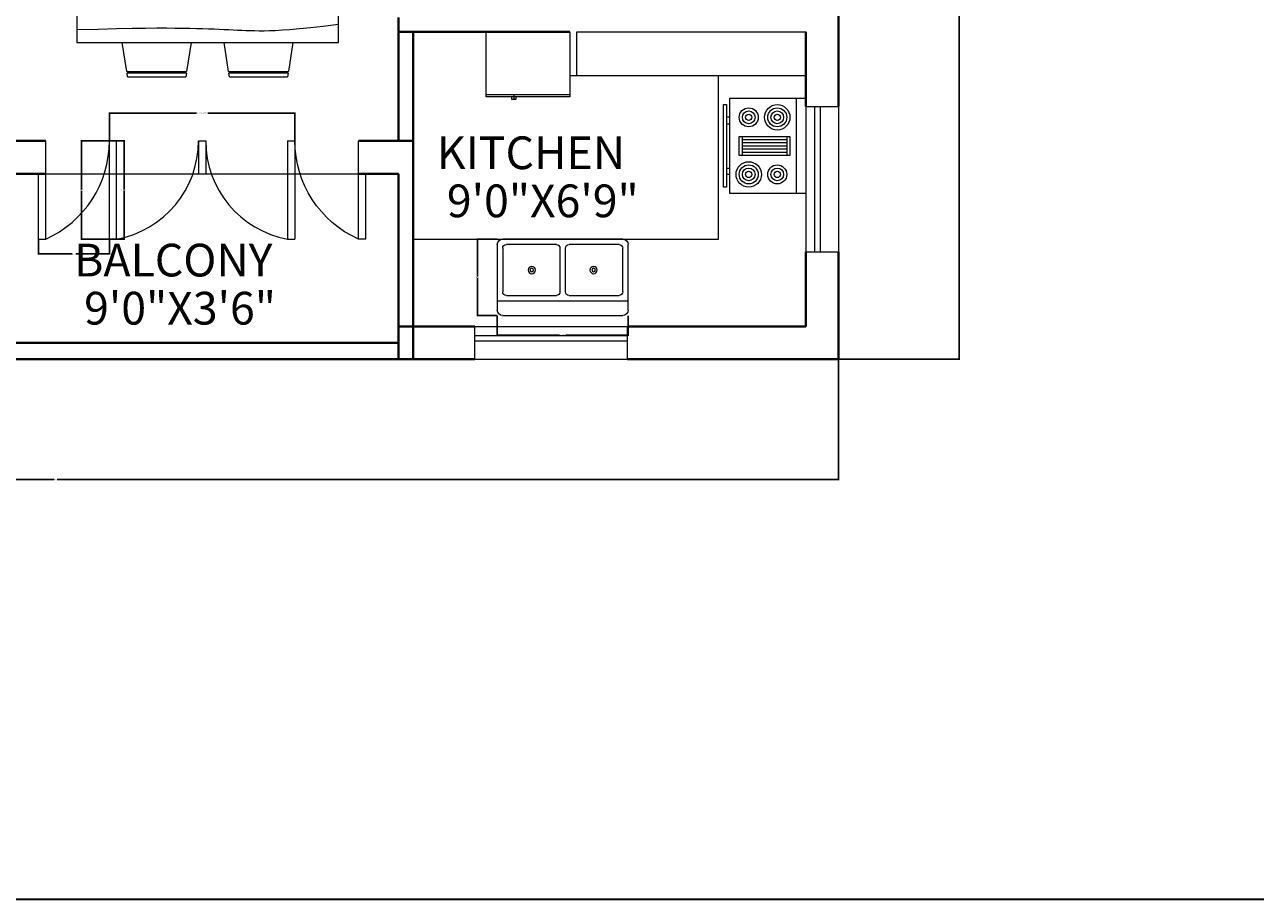
# Model space of a CAD drawing. Units: inches. Extents: x 2220 to 3422, y 783 to 1748.
# Tile 2 of 7: x 2483 to 2821, y 783 to 1023. Entities that reach past the tile are written whole.
import ezdxf

# ---------------------------------------------------------------- set-up
doc = ezdxf.new("R2010")
doc.units = ezdxf.units.IN
for name, color, linetype, lineweight in [('A-ANNO-DIMS', 2, 'Continuous', 18), ('A-ANNO-TTLB', 7, 'Continuous', 35), ('A-AREA-IDEN', 7, 'Continuous', 18), ('A-DOOR', 3, 'Continuous', 20), ('A-EQPM', 9, 'Continuous', 18), ('A-FLOR-CASE', 8, 'Continuous', 18), ('A-FLOR-FIXT', 9, 'Continuous', 18), ('A-FURN', 8, 'Continuous', 18), ('A-GLAZ', 4, 'Continuous', 18), ('A-WALL', 7, 'Continuous', 40)]:
    doc.layers.add(name, color=color, linetype=linetype, lineweight=lineweight)
doc.styles.get("Standard").update_dxf_attribs({"font": 'arial.ttf'})
doc.dimstyles.get("Standard").update_dxf_attribs({"dimtxt": 0.18, "dimasz": 0.18, "dimexe": 0.18, "dimexo": 0.0625, "dimgap": 0.09, "dimtad": 0, "dimtih": 1, "dimtoh": 1, "dimdec": 4, "dimzin": 0, "dimdsep": 46, "dimtxsty": 'Standard', "dimcen": 0.09, "dimadec": 0, "dimazin": 0, "dimtfac": 1, "dimtdec": 4, "dimtofl": 0, "dimtmove": 0, "dimatfit": 3, "dimfxl": 1, "dimtolj": 1, "dimtzin": 0, "dimarcsym": 0})

# ---------------------------------------------------------------- blocks, each defined once
blk = doc.blocks.new('Range-Oven - 30 in top')
for p, q in [((0, -3), (30, -3)), ((12, -6), (18, -6)), ((13, -20), (13, -6)), ((14, -6), (14, -20)), ((15, -20), (15, -6)), ((16, -6), (16, -20)), ((17, -20), (17, -6)), ((18, -20), (12, -20)), ((6, -24), (6, -25)), ((8, -25), (8, -24)), ((22, -25), (22, -24)), ((24, -24), (24, -25))]:
    blk.add_line(p, q)
for points in [[(0, -24), (0, 0), (30, 0), (30, -24)], [(12, -21), (12, -5), (18, -5), (18, -21)], [(2, -26), (2, -25), (28, -25), (28, -26)]]:
    blk.add_lwpolyline(points, close=True)
for centre, radius in [((6, -9), 4), ((6, -9), 3), ((6, -9), 2), ((24, -9), 3), ((24, -9), 2), ((6, -9), 1), ((24, -9), 1), ((6, -18), 3), ((24, -18), 4), ((24, -18), 3), ((6, -18), 2), ((6, -18), 1), ((24, -18), 2), ((24, -18), 1)]:
    blk.add_circle(centre, radius)
blk = doc.blocks.new('Refrigerator-2 door - 36 in top')
for p, q in [((0, -26.999999), (36, -26.999999)), ((11, -27.999999), (11, -28.999999)), ((11, -28.999999), (13, -28.999999)), ((12, -26.999999), (12, -28.999999)), ((13, -28.999999), (13, -27.999999))]:
    blk.add_line(p, q)
blk.add_lwpolyline([(0, -27.999999), (0, 0), (36, 0), (36, -27.999999)], close=True)
blk = doc.blocks.new('Sink-double - 36 in top')
for p, q in [((-18, -4), (18, -4)), ((-0.75, -18.5), (-0.75, -6.5)), ((0.75, -6.5), (0.75, -18.5))]:
    blk.add_line(p, q)
for points in [[(-16.5, 0), (16.5, 0)], [(-18, -19.5), (-18, -1.5)], [(18, -1.5), (18, -19.5)], [(-16.5, -18.5), (-16.5, -6.5)], [(-15.5, -5.5), (-1.75, -5.5)], [(1.75, -5.5), (15.5, -5.5)], [(16.5, -6.5), (16.5, -18.5)], [(-1.75, -19.5), (-15.5, -19.5)], [(15.5, -19.5), (1.75, -19.5)], [(16.5, -21), (-16.5, -21)]]:
    blk.add_lwpolyline(points)
for centre, radius in [((-8.5, -12.5), 1), ((-8.5, -12.5), 0.5), ((8.5, -12.5), 1), ((8.5, -12.5), 0.5)]:
    blk.add_circle(centre, radius)
for centre, radius, start, end in [((-16.5, -1.5), 1.5, 90, 180), ((16.5, -1.5), 1.5, 0, 90), ((-15.5, -6.5), 1, 90, 180), ((-1.75, -6.5), 1, 0, 90), ((1.75, -6.5), 1, 90, 180), ((15.5, -6.5), 1, 0, 90), ((-16.5, -19.5), 1.5, 180, 270), ((-15.5, -18.5), 1, 180, 270), ((-1.75, -18.5), 1, 270, 0), ((1.75, -18.5), 1, 180, 270), ((15.5, -18.5), 1, 270, 0), ((16.5, -19.5), 1.5, 270, 0)]:
    blk.add_arc(centre, radius, start, end)
blk = doc.blocks.new('Dining Set - 36 x 72 in.')
for p, q in [((-22, 27.5), (-22.1562, 26.50042)), ((-22, 27.5), (-6, 27.5)), ((-5.8437, 26.49966), (-6, 27.5)), ((6, 27.5), (5.8438, 26.50042)), ((6, 27.5), (22, 27.5)), ((22.1563, 26.49966), (22, 27.5)), ((-22.2343, 26.00059), (-23.4847, 17.99762)), ((-22.2304, 26), (-5.7608, 26)), ((-5.8416, 26.5), (-22.1534, 26.5)), ((-4.5152, 17.99762), (-5.7655, 25.99926)), ((5.7657, 26.00059), (4.5153, 17.99762)), ((5.7696, 26), (22.2392, 26)), ((22.1584, 26.5), (5.8466, 26.5)), ((23.4848, 17.99762), (22.2345, 25.99926)), ((36, 18), (-36, 18)), ((-36, 18), (-36, -18)), ((36, -18), (36, 18)), ((-45.5, 8), (-44.5004, 8.15617)), ((-45.5, 8), (-45.5, -8)), ((-44.5, -8.15843), (-44.5, 8.15338)), ((-44.0006, 8.23428), (-35.9976, 9.48474)), ((-44, 8.23041), (-44, -8.23915)), ((44.0006, 8.23428), (35.9976, 9.48474)), ((44, 8.23041), (44, -8.23915)), ((44.5, -8.15843), (44.5, 8.15338)), ((45.5, 8), (44.5005, 8.15617)), ((45.5, 8), (45.5, -8)), ((-44.4997, -8.15631), (-45.5, -8)), ((-35.9976, -9.48476), (-43.9993, -8.2345)), ((35.9976, -9.48476), (43.9993, -8.2345)), ((44.4997, -8.15631), (45.5, -8)), ((-36, -18), (36, -18)), ((-22.2343, -26.0006), (-23.4847, -17.99762)), ((-4.5152, -17.99762), (-5.7655, -25.99928)), ((5.7657, -26.0006), (4.5153, -17.99762)), ((23.4848, -17.99762), (22.2345, -25.99928)), ((-22.2304, -26), (-5.7608, -26)), ((-22, -27.5), (-22.1562, -26.50044)), ((-5.8416, -26.5), (-22.1534, -26.5)), ((-5.8437, -26.49967), (-6, -27.5)), ((5.7696, -26), (22.2392, -26)), ((6, -27.5), (5.8438, -26.50044)), ((22.1584, -26.5), (5.8466, -26.5)), ((22.1563, -26.49967), (22, -27.5)), ((-22, -27.5), (-6, -27.5)), ((6, -27.5), (22, -27.5))]:
    blk.add_line(p, q)
for points in [[(-36, 15), (-31.1772, 14.97754), (-26.8079, 14.91406), (-22.8538, 14.81543), (-19.276, 14.6875), (-16.0362, 14.53613), (-13.0957, 14.36718), (-10.4159, 14.18652), (-7.9583, 14), (-5.6904, 13.81315), (-3.6035, 13.63021), (-1.6954, 13.45508), (0.0365, 13.29166), (1.5945, 13.14388), (2.9811, 13.01562), (4.1988, 12.9108), (5.25, 12.83333), (6.1393, 12.78613), (6.8802, 12.76823), (7.4883, 12.77767), (7.9792, 12.8125), (8.3685, 12.87077), (8.6719, 12.95052), (8.9049, 13.0498), (9.0833, 13.16666), (9.2205, 13.29899), (9.3216, 13.44401), (9.3895, 13.59879), (9.4271, 13.76041), (9.4373, 13.92594), (9.4232, 14.09245), (9.3875, 14.257), (9.3333, 14.41666), (9.2638, 14.56917), (9.1836, 14.71484), (9.0975, 14.85465), (9.0104, 14.98958), (8.9272, 15.1206), (8.8529, 15.2487), (8.7922, 15.37483), (8.75, 15.5), (8.7305, 15.62467), (8.7344, 15.74739), (8.7617, 15.86621), (8.8125, 15.97916), (8.8867, 16.08431), (8.9844, 16.17968), (9.1055, 16.26334), (9.25, 16.33333), (9.4189, 16.38802), (9.6172, 16.42708), (9.8506, 16.45052), (10.125, 16.45833), (10.4463, 16.45052), (10.8203, 16.42708), (11.2529, 16.38802), (11.75, 16.33333), (12.3184, 16.26318), (12.9694, 16.17838), (13.7151, 16.07991), (14.5677, 15.96875), (15.5395, 15.84586), (16.6426, 15.71224), (17.8893, 15.56884), (19.2917, 15.41666), (20.859, 15.25667), (22.5879, 15.08984), (24.4721, 14.91715), (26.5052, 14.73958), (28.6809, 14.5581), (30.9929, 14.3737), (33.4347, 14.18733), (36, 14)], [(-36, 10), (-28.9766, 10.14274), (-23.1725, 10.20442), (-18.4241, 10.19775), (-14.5677, 10.13541), (-11.4399, 10.03011), (-8.877, 9.89453), (-6.7154, 9.74137), (-4.7917, 9.58333), (-2.9698, 9.43082), (-1.2246, 9.28515), (0.4415, 9.14534), (2.026, 9.01041), (3.5266, 8.87939), (4.9408, 8.7513), (6.266, 8.62516), (7.5, 8.5), (8.6411, 8.37549), (9.6914, 8.2539), (10.6538, 8.13818), (11.5312, 8.03125), (12.3267, 7.93603), (13.043, 7.85547), (13.6831, 7.79248), (14.25, 7.75), (14.7471, 7.7303), (15.1797, 7.73307), (15.5537, 7.75732), (15.875, 7.80208), (16.1494, 7.86637), (16.3828, 7.94922), (16.5811, 8.04964), (16.75, 8.16666), (16.8944, 8.29915), (17.0143, 8.44531), (17.1089, 8.60319), (17.1771, 8.77083), (17.218, 8.94629), (17.2305, 9.1276), (17.2137, 9.31282), (17.1667, 9.5), (17.0895, 9.6875), (16.987, 9.875), (16.8649, 10.0625), (16.7292, 10.25), (16.5856, 10.4375), (16.4401, 10.625), (16.2985, 10.8125), (16.1667, 11), (16.05, 11.18733), (15.9518, 11.3737), (15.8752, 11.5581), (15.8229, 11.73958), (15.798, 11.91715), (15.8034, 12.08984), (15.842, 12.25667), (15.9167, 12.41666), (16.0295, 12.56836), (16.1784, 12.70833), (16.3605, 12.83268), (16.5729, 12.9375), (16.8127, 13.01888), (17.0768, 13.07291), (17.3625, 13.0957), (17.6667, 13.08333), (17.9894, 13.03312), (18.3418, 12.94726), (18.7382, 12.82918), (19.1927, 12.68229), (19.7195, 12.51001), (20.3327, 12.31575), (21.0465, 12.10294), (21.875, 11.875), (22.8357, 11.63354), (23.959, 11.37304), (25.2786, 11.08618), (26.8282, 10.76562), (28.6414, 10.40405), (30.752, 9.99414), (33.1936, 9.52856), (36, 9)], [(-36, 5.5), (-30.7157, 5.3348), (-26.069, 5.20963), (-21.9946, 5.11767), (-18.4271, 5.05208), (-15.3009, 5.00602), (-12.5508, 4.97265), (-10.1112, 4.94515), (-7.9167, 4.91666), (-5.909, 4.88167), (-4.0586, 4.83984), (-2.3429, 4.79215), (-0.7396, 4.73958), (0.7739, 4.6831), (2.22, 4.6237), (3.6213, 4.56233), (5, 4.5), (6.373, 4.43782), (7.7344, 4.3776), (9.0723, 4.32129), (10.375, 4.27083), (11.6309, 4.22819), (12.8281, 4.19531), (13.9551, 4.17415), (15, 4.16666), (15.954, 4.17448), (16.819, 4.19791), (17.6001, 4.23698), (18.3021, 4.29166), (18.9299, 4.36198), (19.4883, 4.44791), (19.9823, 4.54948), (20.4167, 4.66666), (20.7969, 4.79899), (21.1302, 4.94401), (21.4245, 5.09879), (21.6875, 5.26041), (21.9271, 5.42594), (22.1511, 5.59245), (22.3672, 5.757), (22.5834, 5.91666), (22.8065, 6.06868), (23.0404, 6.21093), (23.2879, 6.34147), (23.5521, 6.45833), (23.8358, 6.55957), (24.142, 6.64323), (24.4735, 6.70735), (24.8334, 6.75), (25.2235, 6.76969), (25.642, 6.76692), (26.0858, 6.74267), (26.5521, 6.69791), (27.0379, 6.63362), (27.5404, 6.55078), (28.0565, 6.45036), (28.5834, 6.33333), (29.1242, 6.19987), (29.7071, 6.04687), (30.3661, 5.87044), (31.1354, 5.66666), (32.0493, 5.43164), (33.142, 5.16146), (34.4475, 4.85221), (36, 4.5)], [(-36, -1), (-30.7915, -0.6591), (-26.0195, -0.38216), (-21.6519, -0.16284), (-17.6563, 0.00521), (-14.0005, 0.12833), (-10.6523, 0.21289), (-7.5796, 0.26522), (-4.75, 0.29166), (-2.134, 0.29793), (0.2878, 0.28711), (2.5317, 0.26163), (4.6146, 0.22396), (6.5529, 0.17651), (8.3633, 0.12174), (10.0623, 0.06209), (11.6667, 0), (13.1899, -0.06201), (14.6341, -0.1211), (15.9982, -0.17432), (17.2813, -0.21875), (18.4823, -0.25147), (19.6003, -0.26953), (20.6343, -0.27002), (21.5834, -0.25), (22.4481, -0.20768), (23.2357, -0.14584), (23.9549, -0.06836), (24.6146, 0.02083), (25.2235, 0.11784), (25.7904, 0.21875), (26.3241, 0.31966), (26.8334, 0.41666), (27.3265, 0.50618), (27.8099, 0.58593), (28.2894, 0.65397), (28.7709, 0.70833), (29.2601, 0.74707), (29.763, 0.76823), (30.2855, 0.76985), (30.8334, 0.75), (31.4088, 0.70784), (31.9994, 0.64713), (32.589, 0.57275), (33.1615, 0.48958), (33.7008, 0.4025), (34.1908, 0.3164), (34.6153, 0.23616), (34.9584, 0.16666), (35.2099, 0.11165), (35.3848, 0.07031), (35.504, 0.04069), (35.5886, 0.02083), (35.6594, 0.00879), (35.7377, 0.0026), (35.8442, 0.00032), (36, 0)], [(-36, -6.5), (-27.1843, -6.31267), (-20.084, -6.1263), (-14.469, -5.9419), (-10.1094, -5.76042), (-6.7752, -5.58285), (-4.2363, -5.41016), (-2.2629, -5.24333), (-0.625, -5.08334), (0.8708, -4.93099), (2.2715, -4.78646), (3.5872, -4.64974), (4.8281, -4.52084), (6.0046, -4.39974), (7.127, -4.28646), (8.2053, -4.18099), (9.25, -4.08334), (10.2705, -3.99382), (11.2734, -3.91407), (12.2647, -3.84603), (13.25, -3.79167), (14.2354, -3.75293), (15.2266, -3.73177), (16.2295, -3.73015), (17.25, -3.75), (18.2912, -3.79248), (19.3451, -3.85547), (20.4009, -3.93604), (21.4479, -4.03125), (22.4754, -4.13819), (23.4727, -4.25391), (24.4289, -4.37549), (25.3334, -4.5), (26.1785, -4.62492), (26.9694, -4.74935), (27.7145, -4.87281), (28.4219, -4.99479), (29.1, -5.11483), (29.7572, -5.23242), (30.4016, -5.34709), (31.0417, -5.45834), (31.6837, -5.56437), (32.3262, -5.65821), (32.9658, -5.73153), (33.599, -5.77604), (34.2224, -5.78345), (34.8327, -5.74545), (35.4264, -5.65373), (36, -5.5)], [(-36, -10), (-26.4022, -9.81299), (-18.4675, -9.62891), (-11.9839, -9.45069), (-6.7396, -9.28125), (-2.5226, -9.12354), (0.8789, -8.98047), (3.6769, -8.85498), (6.0833, -8.75), (8.2767, -8.66765), (10.3021, -8.60677), (12.1712, -8.56543), (13.8958, -8.54167), (15.4876, -8.53353), (16.9583, -8.53907), (18.3197, -8.55632), (19.5834, -8.58334), (20.7616, -8.61841), (21.8685, -8.66081), (22.9188, -8.71004), (23.9271, -8.76563), (24.9081, -8.82707), (25.8763, -8.89388), (26.8465, -8.96558), (27.8334, -9.04167), (28.8474, -9.12118), (29.8828, -9.20117), (30.93, -9.27824), (31.9792, -9.34896), (33.0205, -9.40991), (34.0443, -9.45768), (35.0407, -9.48885), (36, -9.5)], [(-36, -14.5), (-30.0881, -14.33513), (-25.0332, -14.21224), (-20.7312, -14.12647), (-17.0781, -14.07292), (-13.97, -14.04671), (-11.3027, -14.04297), (-8.9724, -14.05681), (-6.875, -14.08334), (-4.9224, -14.11833), (-3.0905, -14.16016), (-1.3709, -14.20785), (0.2448, -14.26042), (1.7647, -14.3169), (3.1973, -14.3763), (4.5507, -14.43767), (5.8333, -14.5), (7.0554, -14.5621), (8.235, -14.62175), (9.3922, -14.67652), (10.5469, -14.72396), (11.7192, -14.76164), (12.929, -14.78711), (14.1965, -14.79794), (15.5417, -14.79167), (16.9933, -14.76424), (18.6152, -14.70508), (20.4804, -14.60197), (22.6615, -14.44271), (25.2312, -14.21509), (28.2624, -13.9069), (31.8277, -13.50594), (36, -13)]]:
    blk.add_lwpolyline(points)
blk = doc.blocks.new('DOOR-BALCONY-CENTER')
for p, q in [((0, 0), (0, 27)), ((0, 27), (2, 27)), ((2, 0), (2, 27)), ((24.5, 27), (24.5, 18)), ((24.5, 27), (26.5, 27)), ((26.5, 27), (26.5, 18)), ((49, 27), (49, 0)), ((49, 27), (51, 27)), ((51, 27), (51, 0)), ((0, 0), (2, 0)), ((49, 0), (51, 0))]:
    blk.add_line(p, q)
for centre, start, end in [((-2.95, 27), 280.3889, 0), ((53.95, 27), 180, 259.6111)]:
    blk.add_arc(centre, 27.45, start, end)
blk = doc.blocks.new('DOOR-BALCONY-END-A')
for p, q in [((2, 0), (2, 27)), ((0, 0), (0, 18)), ((0, 0), (2, 0))]:
    blk.add_line(p, q)
blk.add_arc((-10.08, 27), 29.58, 294.1016, 0)
blk = doc.blocks.new('*D29')
at = {"layer": 'A-ANNO-DIMS', "color": 0, "lineweight": -2, "transparency": 16777216}
for p, q in [((2612.7, 943.33), (2612.7, 937.81)), ((2648.7, 943.33), (2648.7, 937.81)), ((2612.88, 937.99), (2629.85, 937.99)), ((2648.52, 937.99), (2631.56, 937.99))]:
    blk.add_line(p, q, dxfattribs=at)
at = {"layer": 'A-ANNO-DIMS', "color": 0, "transparency": 16777216}
for points in [[(2612.88, 938.02), (2612.88, 937.96), (2612.7, 937.99)], [(2648.52, 938.02), (2648.52, 937.96), (2648.7, 937.99)]]:
    blk.add_solid(points, dxfattribs=at)
at = {"layer": 'Defpoints', "color": 0, "transparency": 16777216}
for p in [(2612.7, 943.39), (2648.7, 943.39), (2648.7, 937.99)]:
    blk.add_point(p, dxfattribs=at)
at = {"layer": 'A-ANNO-DIMS', "color": 0, "transparency": 16777216, "insert": (2630.7, 937.99), "char_height": 0.18, "attachment_point": 5}
blk.add_mtext('\\A1;SINK 36 TYP.', dxfattribs=at)
blk = doc.blocks.new('*D30')
at = {"layer": 'A-ANNO-DIMS', "color": 0, "lineweight": -2, "transparency": 16777216}
for p, q in [((2612.64, 964.39), (2607.12, 964.39)), ((2607.3, 964.21), (2607.3, 954.07)), ((2607.3, 943.57), (2607.3, 953.71)), ((2612.64, 943.39), (2607.12, 943.39))]:
    blk.add_line(p, q, dxfattribs=at)
at = {"layer": 'A-ANNO-DIMS', "color": 0, "transparency": 16777216}
for points in [[(2607.27, 964.21), (2607.33, 964.21), (2607.3, 964.39)], [(2607.27, 943.57), (2607.33, 943.57), (2607.3, 943.39)]]:
    blk.add_solid(points, dxfattribs=at)
at = {"layer": 'Defpoints', "color": 0, "transparency": 16777216}
for p in [(2612.7, 964.39), (2607.3, 943.39), (2612.7, 943.39)]:
    blk.add_point(p, dxfattribs=at)
at = {"layer": 'A-ANNO-DIMS', "color": 0, "transparency": 16777216, "insert": (2607.3, 953.89), "char_height": 0.18, "attachment_point": 5}
blk.add_mtext('\\A1;21 TYP.', dxfattribs=at)
blk = doc.blocks.new('*D43')
at = {"layer": 'A-ANNO-DIMS', "color": 0, "lineweight": -2, "transparency": 16777216}
for p, q in [((2506.05, 991.45), (2506.05, 999.22)), ((2506.23, 999.04), (2529.97, 999.04)), ((2556.87, 999.04), (2533.12, 999.04)), ((2557.05, 991.45), (2557.05, 999.22))]:
    blk.add_line(p, q, dxfattribs=at)
at = {"layer": 'A-ANNO-DIMS', "color": 0, "transparency": 16777216}
for points in [[(2506.23, 999.07), (2506.23, 999.01), (2506.05, 999.04)], [(2556.87, 999.07), (2556.87, 999.01), (2557.05, 999.04)]]:
    blk.add_solid(points, dxfattribs=at)
at = {"layer": 'Defpoints', "color": 0, "transparency": 16777216}
for p in [(2557.05, 999.04), (2506.05, 991.39), (2557.05, 991.39)]:
    blk.add_point(p, dxfattribs=at)
at = {"layer": 'A-ANNO-DIMS', "color": 0, "transparency": 16777216, "insert": (2531.55, 999.04), "char_height": 0.18, "attachment_point": 5}
blk.add_mtext('\\A1;BALCONY DOOR 51 TYP.', dxfattribs=at)
blk = doc.blocks.new('*D44')
at = {"layer": 'A-ANNO-DIMS', "color": 0, "lineweight": -2, "transparency": 16777216}
for p, q in [((2505.98, 991.39), (2498.22, 991.39)), ((2498.4, 991.21), (2498.4, 978.07)), ((2498.4, 964.57), (2498.4, 977.71)), ((2505.98, 964.39), (2498.22, 964.39))]:
    blk.add_line(p, q, dxfattribs=at)
at = {"layer": 'A-ANNO-DIMS', "color": 0, "transparency": 16777216}
for points in [[(2498.37, 991.21), (2498.43, 991.21), (2498.4, 991.39)], [(2498.37, 964.57), (2498.43, 964.57), (2498.4, 964.39)]]:
    blk.add_solid(points, dxfattribs=at)
at = {"layer": 'Defpoints', "color": 0, "transparency": 16777216}
for p in [(2498.4, 991.39), (2506.05, 991.39), (2506.05, 964.39)]:
    blk.add_point(p, dxfattribs=at)
at = {"layer": 'A-ANNO-DIMS', "color": 0, "transparency": 16777216, "insert": (2498.4, 977.89), "char_height": 0.18, "attachment_point": 5}
blk.add_mtext('\\A1;27 TYP.', dxfattribs=at)
blk = doc.blocks.new('*D45')
at = {"layer": 'A-ANNO-DIMS', "color": 0, "lineweight": -2, "transparency": 16777216}
for p, q in [((2506.11, 991.39), (2510.28, 991.39)), ((2510.1, 991.21), (2510.1, 978.07)), ((2510.1, 964.57), (2510.1, 977.71)), ((2506.11, 964.39), (2510.28, 964.39))]:
    blk.add_line(p, q, dxfattribs=at)
at = {"layer": 'A-ANNO-DIMS', "color": 0, "transparency": 16777216}
for points in [[(2510.07, 991.21), (2510.13, 991.21), (2510.1, 991.39)], [(2510.07, 964.57), (2510.13, 964.57), (2510.1, 964.39)]]:
    blk.add_solid(points, dxfattribs=at)
at = {"layer": 'Defpoints', "color": 0, "transparency": 16777216}
for p in [(2506.05, 991.39), (2510.1, 991.39), (2506.05, 964.39)]:
    blk.add_point(p, dxfattribs=at)
at = {"layer": 'A-ANNO-DIMS', "color": 0, "transparency": 16777216, "insert": (2510.1, 977.89), "char_height": 0.18, "attachment_point": 5}
blk.add_mtext('\\A1;END LEAF A 27 TYP.', dxfattribs=at)
blk = doc.blocks.new('*D46')
at = {"layer": 'A-ANNO-DIMS', "color": 0, "lineweight": -2, "transparency": 16777216}
for p, q in [((2486.55, 964.33), (2486.55, 960.16)), ((2506.05, 964.33), (2506.05, 960.16)), ((2486.73, 960.34), (2495.77, 960.34)), ((2505.87, 960.34), (2496.83, 960.34))]:
    blk.add_line(p, q, dxfattribs=at)
at = {"layer": 'A-ANNO-DIMS', "color": 0, "transparency": 16777216}
for points in [[(2486.73, 960.37), (2486.73, 960.31), (2486.55, 960.34)], [(2505.87, 960.37), (2505.87, 960.31), (2506.05, 960.34)]]:
    blk.add_solid(points, dxfattribs=at)
at = {"layer": 'Defpoints', "color": 0, "transparency": 16777216}
for p in [(2486.55, 964.39), (2506.05, 964.39), (2506.05, 960.34)]:
    blk.add_point(p, dxfattribs=at)
at = {"layer": 'A-ANNO-DIMS', "color": 0, "transparency": 16777216, "insert": (2496.3, 960.34), "char_height": 0.18, "attachment_point": 5}
blk.add_mtext('\\A1;20 TYP.', dxfattribs=at)
blk = doc.blocks.new('*D53')
at = {"layer": 'A-ANNO-DIMS', "color": 0, "lineweight": -2, "transparency": 16777216}
for p, q in [((2276.05, 931.33), (2276.05, 898.06)), ((2706.55, 931.33), (2706.55, 898.06)), ((2276.23, 898.24), (2490.9, 898.24)), ((2706.37, 898.24), (2491.69, 898.24))]:
    blk.add_line(p, q, dxfattribs=at)
at = {"layer": 'A-ANNO-DIMS', "color": 0, "transparency": 16777216}
for points in [[(2276.23, 898.27), (2276.23, 898.21), (2276.05, 898.24)], [(2706.37, 898.27), (2706.37, 898.21), (2706.55, 898.24)]]:
    blk.add_solid(points, dxfattribs=at)
at = {"layer": 'Defpoints', "color": 0, "transparency": 16777216}
for p in [(2276.05, 931.39), (2706.55, 931.39), (2706.55, 898.24)]:
    blk.add_point(p, dxfattribs=at)
at = {"layer": 'A-ANNO-DIMS', "color": 0, "transparency": 16777216, "insert": (2491.3, 898.24), "char_height": 0.18, "attachment_point": 5}
blk.add_mtext('\\A1;430.5', dxfattribs=at)
blk = doc.blocks.new('*D57')
at = {"layer": 'A-ANNO-DIMS', "color": 0, "lineweight": -2, "transparency": 16777216}
for p, q in [((2706.61, 1218.39), (2739.88, 1218.39)), ((2739.7, 1218.21), (2739.7, 1075.07)), ((2739.7, 931.57), (2739.7, 1074.71)), ((2706.61, 931.39), (2739.88, 931.39))]:
    blk.add_line(p, q, dxfattribs=at)
at = {"layer": 'A-ANNO-DIMS', "color": 0, "transparency": 16777216}
for points in [[(2739.67, 1218.21), (2739.73, 1218.21), (2739.7, 1218.39)], [(2739.67, 931.57), (2739.73, 931.57), (2739.7, 931.39)]]:
    blk.add_solid(points, dxfattribs=at)
at = {"layer": 'Defpoints', "color": 0, "transparency": 16777216}
for p in [(2706.55, 1218.39), (2706.55, 931.39), (2739.7, 931.39)]:
    blk.add_point(p, dxfattribs=at)
at = {"layer": 'A-ANNO-DIMS', "color": 0, "transparency": 16777216, "insert": (2739.7, 1074.89), "char_height": 0.18, "attachment_point": 5}
blk.add_mtext('\\A1;287', dxfattribs=at)

msp = doc.modelspace()

# ---------------------------------------------------------------- linework, layer by layer
at = {"layer": 'A-ANNO-TTLB'}
msp.add_lwpolyline([(2220.0037, 1747.9465), (3422.343, 1747.9465), (3422.343, 782.804), (2220.0037, 782.804)], close=True, dxfattribs=at)
at = {"layer": 'A-DOOR'}
msp.add_line((2488.5466, 982.3907), (2574.5466, 982.3907), dxfattribs=at)
at = {"layer": 'A-FLOR-CASE'}
for p, q in [((2632.6148, 1021.3907), (2632.6148, 1009.3907)), ((2634.5466, 1009.3907), (2634.5466, 1021.3907)), ((2634.5466, 1021.3907), (2697.5466, 1021.3907)), ((2632.6148, 1009.3907), (2697.5466, 1009.3907)), ((2673.5466, 964.3907), (2673.5466, 1009.3907)), ((2589.5466, 964.3907), (2673.5466, 964.3907))]:
    msp.add_line(p, q, dxfattribs=at)
at = {"layer": 'A-GLAZ'}
for p, q in [((2697.5466, 1000.8907), (2706.5466, 1000.8907)), ((2697.5466, 1000.8907), (2697.5466, 960.8907)), ((2700.0466, 960.8907), (2700.0466, 1000.8907)), ((2701.5466, 960.8907), (2701.5466, 1000.8907)), ((2706.5466, 1000.8907), (2706.5466, 960.8907)), ((2697.5466, 960.8907), (2706.5466, 960.8907)), ((2606.5466, 931.3907), (2606.5466, 940.3907)), ((2606.5466, 940.3907), (2648.5466, 940.3907)), ((2606.5466, 937.8907), (2648.5466, 937.8907)), ((2648.5466, 931.3907), (2648.5466, 940.3907)), ((2606.5466, 936.3907), (2648.5466, 936.3907)), ((2606.5466, 931.3907), (2648.5466, 931.3907))]:
    msp.add_line(p, q, dxfattribs=at)
at = {"layer": 'A-WALL'}
for p, q in [((2706.5466, 1000.8907), (2706.5466, 1037.3907)), ((2585.5466, 1021.3907), (2585.5466, 1025.3907)), ((2585.5466, 1021.3907), (2632.6148, 1021.3907)), ((2585.5466, 1021.3907), (2585.5466, 991.3907)), ((2589.5466, 991.3907), (2589.5466, 1021.3907)), ((2697.5466, 1000.8907), (2697.5466, 1021.3907)), ((2477.5466, 991.3907), (2488.5466, 991.3907)), ((2574.5466, 991.3907), (2589.5466, 991.3907)), ((2589.5466, 931.3907), (2589.5466, 991.3907)), ((2477.5466, 982.3907), (2488.5466, 982.3907)), ((2574.5466, 982.3907), (2585.5466, 982.3907)), ((2585.5466, 931.3907), (2585.5466, 982.3907)), ((2697.5466, 940.3907), (2697.5466, 960.8907)), ((2706.5466, 931.3907), (2706.5466, 960.8907)), ((2585.5466, 940.3907), (2606.5466, 940.3907)), ((2648.5466, 940.3907), (2697.5466, 940.3907)), ((2477.5466, 935.8907), (2585.5466, 935.8907)), ((2477.5466, 931.3907), (2585.5466, 931.3907)), ((2585.5466, 931.3907), (2589.5466, 931.3907)), ((2589.5466, 931.3907), (2606.5466, 931.3907)), ((2648.5466, 931.3907), (2706.5466, 931.3907))]:
    msp.add_line(p, q, dxfattribs=at)

# ---------------------------------------------------------------- block references
at = {"layer": 'A-DOOR'}
for name, p in [('DOOR-BALCONY-END-A', (2486.547, 964.391)), ('DOOR-BALCONY-CENTER', (2506.047, 964.391))]:
    msp.add_blockref(name, p, dxfattribs=at)
at = {"layer": 'A-DOOR', "extrusion": (0, 0, -1), "zscale": -1}
msp.add_blockref('DOOR-BALCONY-END-A', (-2576.5463, 964.391), dxfattribs=at)
at = {"layer": 'A-EQPM', "xscale": 0.6390408655968428, "yscale": 0.6390408655968428, "zscale": 0.6390408655968428}
msp.add_blockref('Refrigerator-2 door - 36 in top', (2609.6093, 1021.3907), dxfattribs=at)
at = {"layer": 'A-EQPM', "xscale": 0.8722005701805317, "yscale": 0.8722005701805317, "zscale": 0.8722005701805317, "rotation": 270}
msp.add_blockref('Range-Oven - 30 in top', (2697.5473, 1003.1234), dxfattribs=at)
at = {"layer": 'A-FLOR-FIXT', "xscale": -1, "rotation": 180}
msp.add_blockref('Sink-double - 36 in top', (2630.7033, 943.3898), dxfattribs=at)
at = {"layer": 'A-FURN'}
msp.add_blockref('Dining Set - 36 x 72 in.', (2533.0492, 1036.5138), dxfattribs=at)

# ---------------------------------------------------------------- texts
at = {"layer": 'A-AREA-IDEN'}
for s, p in [('KITCHEN', (2596.0924, 983.6423)), (' 9\'0"X6\'9"', (2596.0924, 970.4153)), ('BALCONY', (2496.3387, 954.1225)), (' 9\'0"X3\'6"', (2496.3387, 940.8954))]:
    msp.add_text(s, height=9, dxfattribs=at).set_placement(p)

# ---------------------------------------------------------------- dimensions: what is measured, and where the dimension line sits
at = {"layer": 'A-ANNO-DIMS'}
dim = msp.add_linear_dim(base=(2739.6966, 931.3907), p1=(2706.5466, 1218.3907), p2=(2706.5466, 931.3907), angle=90, dimstyle='Standard', override={"dimdec": 0, "dimlfac": 1, "dimrnd": 0, "dimzin": 0, "dimdsep": 46, "dimlunit": 2}, dxfattribs=at)
dim.commit()
dim.dimension.update_dxf_attribs({"geometry": '*D57', "text_midpoint": (2739.6966, 1074.8907)})
for base, p1, p2, text, picture, middle in [((2557.0466, 999.0407), (2506.0466, 991.3907), (2557.0466, 991.3907), 'BALCONY DOOR <> TYP.', '*D43', (2531.5466, 999.0407)), ((2506.0466333189, 960.3406899565), (2486.5466333189, 964.3906899565), (2506.0466333189, 964.3906899565), '<> TYP.', '*D46', (2496.2966333189, 960.3406899565)), ((2648.7033, 937.9898), (2612.7033, 943.3898), (2648.7033, 943.3898), 'SINK <> TYP.', '*D29', (2630.7033, 937.9898))]:
    dim = msp.add_linear_dim(base=base, p1=p1, p2=p2, text=text, dimstyle='Standard', override={"dimdec": 0, "dimlfac": 1, "dimrnd": 0, "dimzin": 0, "dimdsep": 46, "dimlunit": 2}, dxfattribs=at)
    dim.commit()
    dim.dimension.update_dxf_attribs({"geometry": picture, "text_midpoint": middle})
for base, p1, p2, angle, text, picture, middle in [((2498.3966, 991.3907), (2506.0466, 964.3907), (2506.0466, 991.3907), 90, '<> TYP.', '*D44', (2498.3966, 977.8907)), ((2510.0966, 991.3907), (2506.0466, 964.3907), (2506.0466, 991.3907), 90, 'END LEAF A <> TYP.', '*D45', (2510.0966, 977.8907)), ((2607.3033, 943.3898), (2612.7033, 964.3898), (2612.7033, 943.3898), 270, '<> TYP.', '*D30', (2607.3033, 953.8898))]:
    dim = msp.add_linear_dim(base=base, p1=p1, p2=p2, angle=angle, text=text, dimstyle='Standard', override={"dimdec": 0, "dimlfac": 1, "dimrnd": 0, "dimzin": 0, "dimdsep": 46, "dimlunit": 2}, dxfattribs=at)
    dim.commit()
    dim.dimension.update_dxf_attribs({"geometry": picture, "text_midpoint": middle})
dim = msp.add_linear_dim(base=(2706.5466, 898.2407), p1=(2276.0466, 931.3907), p2=(2706.5466, 931.3907), dimstyle='Standard', override={"dimdec": 1, "dimlfac": 1, "dimrnd": 0, "dimzin": 0, "dimdsep": 46, "dimlunit": 2}, dxfattribs=at)
dim.commit()
dim.dimension.update_dxf_attribs({"geometry": '*D53', "text_midpoint": (2491.2966, 898.2407)})

doc.saveas('drawing.dxf')
